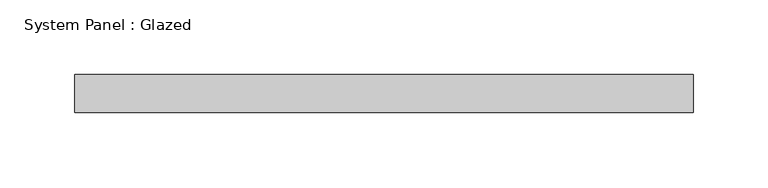
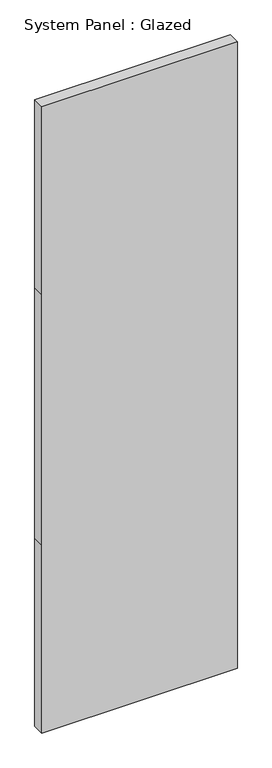
"""IFC4 building model written with IfcOpenShell, lengths in millimetres: plate geometry, System Panel : Glazed."""

from ifc_helpers import new_model, si_unit, frame, origin, place, context, project, spatial, polyline, outline, extrude, source, transform, mapped, element, save


def system_panel_glazed_aa4e1581(model_context):
    return source(origin(), model_context, "Body", "SweptSolid", [
        extrude(outline(polyline([(0.0, -206.375), (0.0, 206.375), (419.1, 206.375), (977.9, 206.375), (1397.0, 206.375), (1397.0, -206.375), (977.9, -206.375), (419.1, -206.375), (0.0, -206.375)])), frame((0.0, 19.05, 0.0), z_axis=(0.0, 1.0, 0.0), x_axis=(0.0, 0.0, 1.0)), (0.0, 0.0, 1.0), 25.4),
    ])


if __name__ == "__main__":
    model = new_model("IFC4")
    model_context = context("Model", 3, world=origin())
    ifc_project = project(units=[si_unit("LENGTHUNIT", "METRE", prefix="MILLI")], contexts=[model_context])
    site = spatial("IfcSite", under=ifc_project)
    building = spatial("IfcBuilding", under=site)
    placement = place(None, origin())
    system_panel_glazed_shape = system_panel_glazed_aa4e1581(model_context)
    element("IfcPlate", 1, ObjectType="System Panel : Glazed", at=placement, inside=building, context=model_context, shape_type="MappedRepresentation", body=[
        mapped(system_panel_glazed_shape, transform((0.0, 0.0, 0.0), x_axis=(1.0, 0.0, 0.0), y_axis=(0.0, 1.0, 0.0), z_axis=(0.0, 0.0, 1.0))),
    ])
    save(model, "model.ifc")

# Revit data of these elements
# Type "System Panel : Glazed"
#   Construction Type Id = "GSP4R"
#   Analytic Construction = "1/8 in Pilkington single glazing"
#   Visual Light Transmittance = 0.9
#   Solar Heat Gain Coefficient = 0.86
#   Heat Transfer Coefficient (U) = 1.18115 BTU/(h·ft²·°F)
#   Define Thermal Properties by = 1
# Element 1 (IfcPlate, "System Panel : Glazed")
#   Materials on its faces: "Glass"
# Materials
#   "Glass": class "Glass", colour RGB 0 128 192, transparency 0.75, Description = "Soda Lime Glass", Cost = 0
